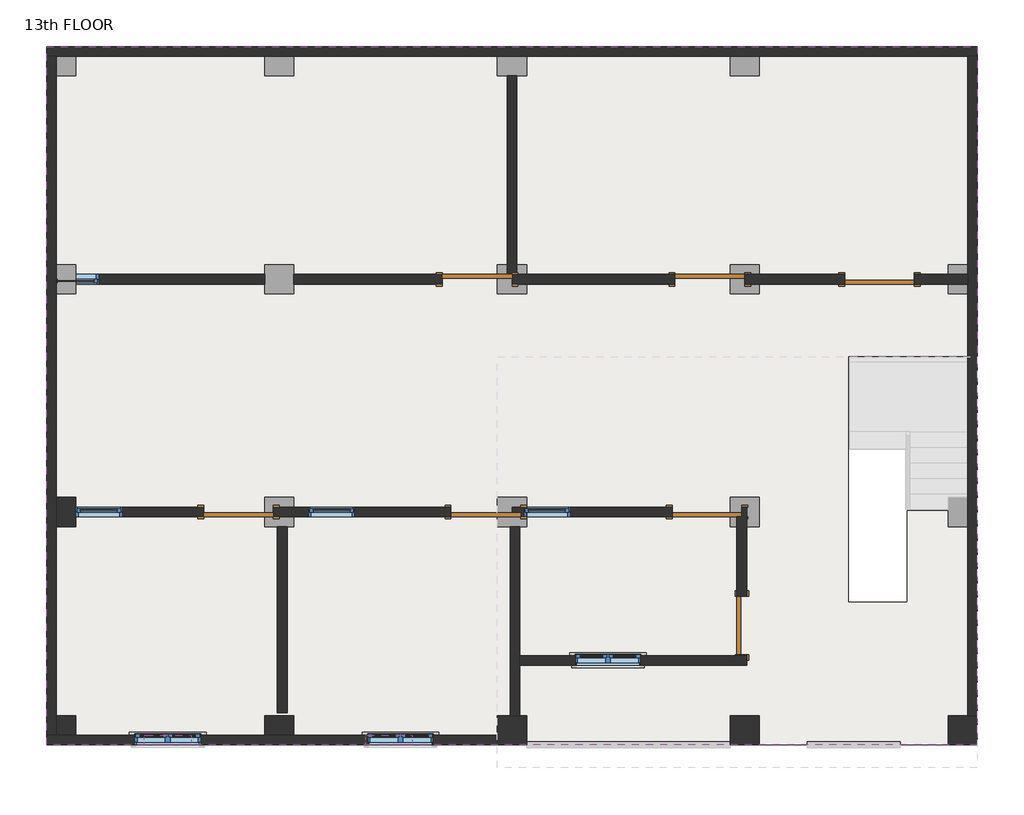
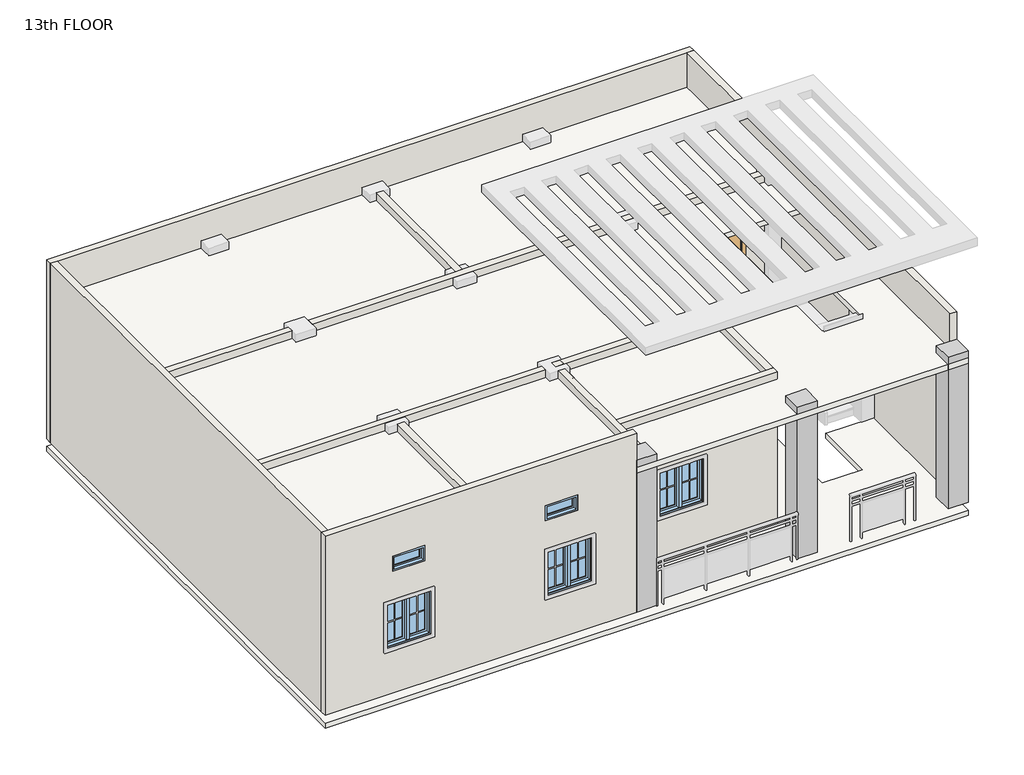
# One storey, part 1 of 2: 15 walls, 9 windows, 7 doors, 6 columns, 2 slabs.
"""IFC4 building model written with IfcOpenShell, lengths in millimetres."""

from ifc_helpers import new_model, si_unit, frame, origin, place, context, project, spatial, polyline, outline, extrude, faceted_brep, transform, mapped, element, save
from components import door_e00f436c, door_a1797ceb, window_4c2727af, window_0bf3737e, window_78893e6c, window_0d9958e7

model = new_model("IFC4")

# Units and contexts
model_context = context("Model", 3, world=origin())
ifc_project = project(units=[si_unit("LENGTHUNIT", "METRE", prefix="MILLI")], contexts=[model_context])

# Site, building, storey
site = spatial("IfcSite", under=ifc_project)
building = spatial("IfcBuilding", under=site)
storey = spatial("IfcBuildingStorey", under=building, Name="13th FLOOR", Elevation=39471.6)

# Columns
placement = place(None, origin())
element("IfcColumn", 1, ObjectType="column family : column family", at=placement, inside=storey, context=model_context, shape_type="SweptSolid", body=[
    extrude(outline(polyline([(-15433.597125, 2867.2065522), (-15433.597125, 2486.2065522), (-15687.597125, 2486.2065522), (-15687.597125, 2867.2065522), (-15433.597125, 2867.2065522)])), frame((0.0, 0.0, 39476.6), z_axis=(0.0, 0.0, 1.0), x_axis=(1.0, 0.0, 0.0)), (0.0, 0.0, 1.0), 3038.0),
])
element("IfcColumn", 2, ObjectType="column family : column family", at=placement, inside=storey, context=model_context, shape_type="SweptSolid", body=[
    extrude(outline(polyline([(-15433.597125, 9.7065522), (-15433.597125, -244.2934478), (-15687.597125, -244.2934478), (-15687.597125, 9.7065522), (-15433.597125, 9.7065522)])), frame((0.0, 0.0, 39476.6), z_axis=(0.0, 0.0, 1.0), x_axis=(1.0, 0.0, 0.0)), (0.0, 0.0, 1.0), 3038.0),
])
element("IfcColumn", 3, ObjectType="column family : column family", at=placement, inside=storey, context=model_context, shape_type="SweptSolid", body=[
    extrude(outline(polyline([(-3622.597125, 9.7065522), (-3622.597125, -371.2934478), (-4003.597125, -371.2934478), (-4003.597125, 9.7065522), (-3622.597125, 9.7065522)])), frame((0.0, 0.0, 39476.6), z_axis=(0.0, 0.0, 1.0), x_axis=(1.0, 0.0, 0.0)), (0.0, 0.0, 1.0), 3038.0),
])
element("IfcColumn", 4, ObjectType="column family : column family", at=placement, inside=storey, context=model_context, shape_type="SweptSolid", body=[
    extrude(outline(polyline([(-6480.097125, 9.7065522), (-6480.097125, -371.2934478), (-6861.097125, -371.2934478), (-6861.097125, 9.7065522), (-6480.097125, 9.7065522)])), frame((0.0, 0.0, 39476.6), z_axis=(0.0, 0.0, 1.0), x_axis=(1.0, 0.0, 0.0)), (0.0, 0.0, 1.0), 3038.0),
])
element("IfcColumn", 5, ObjectType="column family : column family", at=placement, inside=storey, context=model_context, shape_type="SweptSolid", body=[
    extrude(outline(polyline([(-9528.097125, 9.7065522), (-9528.097125, -371.2934478), (-9909.097125, -371.2934478), (-9909.097125, 9.7065522), (-9528.097125, 9.7065522)])), frame((0.0, 0.0, 39476.6), z_axis=(0.0, 0.0, 1.0), x_axis=(1.0, 0.0, 0.0)), (0.0, 0.0, 1.0), 3038.0),
])
element("IfcColumn", 6, ObjectType="column family : column family", at=placement, inside=storey, context=model_context, shape_type="SweptSolid", body=[
    extrude(outline(polyline([(-12957.097125, 9.7065522), (-12576.097125, 9.7065522), (-12576.097125, -244.2934478), (-12957.097125, -244.2934478), (-12957.097125, 9.7065522)])), frame((0.0, 0.0, 39476.6), z_axis=(0.0, 0.0, 1.0), x_axis=(1.0, 0.0, 0.0)), (0.0, 0.0, 1.0), 3038.0),
])

# Doors
door_shape = door_e00f436c(model_context)
element("IfcDoor", 7, ObjectType="Single-Flush : 30\" x 80\"", at=placement, inside=storey, context=model_context, shape_type="MappedRepresentation", body=[
    mapped(door_shape, transform((-6708.697125, 1190.8065522, 39471.6), x_axis=(0.0, -1.0, 0.0), y_axis=(1.0, 0.0, 0.0), z_axis=(0.0, 0.0, 1.0))),
])
door_2_shape = door_a1797ceb(model_context)
element("IfcDoor", 8, ObjectType="Single-Flush : 36\" x 84\"", at=placement, inside=storey, context=model_context, shape_type="MappedRepresentation", body=[
    mapped(door_2_shape, transform((-10175.797125, 5724.7065522, 39471.6), x_axis=(1.0, 0.0, 0.0), y_axis=(0.0, 1.0, 0.0), z_axis=(0.0, 0.0, 1.0))),
])
element("IfcDoor", 9, ObjectType="Single-Flush : 36\" x 84\"", at=placement, inside=storey, context=model_context, shape_type="MappedRepresentation", body=[
    mapped(door_2_shape, transform((-10061.497125, 2676.7065522, 39471.6), x_axis=(-1.0, 0.0, 0.0), y_axis=(0.0, -1.0, 0.0), z_axis=(0.0, 0.0, 1.0))),
])
element("IfcDoor", 10, ObjectType="Single-Flush : 36\" x 84\"", at=placement, inside=storey, context=model_context, shape_type="MappedRepresentation", body=[
    mapped(door_2_shape, transform((-13299.997125, 2676.7065522, 39471.6), x_axis=(-1.0, 0.0, 0.0), y_axis=(0.0, -1.0, 0.0), z_axis=(0.0, 0.0, 1.0))),
])
element("IfcDoor", 11, ObjectType="Single-Flush : 36\" x 84\"", at=placement, inside=storey, context=model_context, shape_type="MappedRepresentation", body=[
    mapped(door_2_shape, transform((-7127.797125, 5724.7065522, 39471.6), x_axis=(1.0, 0.0, 0.0), y_axis=(0.0, 1.0, 0.0), z_axis=(0.0, 0.0, 1.0))),
])
element("IfcDoor", 12, ObjectType="Single-Flush : 36\" x 84\"", at=placement, inside=storey, context=model_context, shape_type="MappedRepresentation", body=[
    mapped(door_2_shape, transform((-7165.897125, 2676.7065522, 39471.6), x_axis=(-1.0, 0.0, 0.0), y_axis=(0.0, -1.0, 0.0), z_axis=(0.0, 0.0, 1.0))),
])
element("IfcDoor", 13, ObjectType="Single-Flush : 36\" x 84\"", at=placement, inside=storey, context=model_context, shape_type="MappedRepresentation", body=[
    mapped(door_2_shape, transform((-4905.297125, 5724.7065522, 39471.6), x_axis=(-1.0, 0.0, 0.0), y_axis=(0.0, -1.0, 0.0), z_axis=(0.0, 0.0, 1.0))),
])

# Slabs
element("IfcSlab", 14, ObjectType="Generic - 4\"", at=placement, inside=storey, context=model_context, shape_type="SweptSolid", body=[
    extrude(outline(polyline([(-3622.597125, 8772.7065522), (-3622.597125, -371.2934478), (-15814.597125, -371.2934478), (-15814.597125, 8772.7065522), (-3622.597125, 8772.7065522)]), holes=[polyline([(-3734.357125, 4711.0719226), (-5310.2646464, 4711.0719226), (-5310.2646464, 1502.3126957), (-4547.7736682, 1502.3126957), (-4547.7736682, 2699.911213), (-3734.357125, 2699.911213), (-3734.357125, 4711.0719226)])]), frame((0.0, 0.0, 39217.6), z_axis=(0.0, 0.0, 1.0), x_axis=(1.0, 0.0, 0.0)), (0.0, 0.0, 1.0), 101.6),
])
element("IfcSlab", 15, ObjectType="Generic - 4\"", at=placement, inside=storey, context=model_context, shape_type="SweptSolid", body=[
    extrude(outline(polyline([(-3622.597125, 8772.7065522), (-3622.597125, -371.2934478), (-15814.597125, -371.2934478), (-15814.597125, 8772.7065522), (-3622.597125, 8772.7065522)]), holes=[polyline([(-3734.357125, 4711.0719226), (-5310.2646464, 4711.0719226), (-5310.2646464, 1502.3126957), (-4547.7736682, 1502.3126957), (-4547.7736682, 2699.911213), (-3734.357125, 2699.911213), (-3734.357125, 4711.0719226)])]), frame((0.0, 0.0, 42265.6), z_axis=(0.0, 0.0, 1.0), x_axis=(1.0, 0.0, 0.0)), (0.0, 0.0, 1.0), 101.6),
])

# Walls
element("IfcWall", 16, ObjectType="Generic - 5\"", at=placement, inside=storey, context=model_context, shape_type="Brep", body=[
    faceted_brep([(-15814.597125, 8645.7065522, 39471.6), (-15687.597125, 8645.7065522, 39471.6), (-3749.597125, 8645.7065522, 39471.6), (-3622.597125, 8645.7065522, 39471.6), (-3622.597125, 8645.7065522, 43063.6342883), (-3749.597125, 8645.7065522, 43063.6342883), (-15687.597125, 8645.7065522, 43063.6342883), (-15814.597125, 8645.7065522, 43063.6342883), (-15814.597125, 8772.7065522, 39471.6), (-15814.597125, 8772.7065522, 43063.6342883), (-3622.597125, 8772.7065522, 43063.6342883), (-3622.597125, 8772.7065522, 39471.6)], [[[0, 1, 2, 3, 4, 5, 6, 7]], [[8, 9, 10, 11]], [[3, 2, 1, 0, 8, 11]], [[7, 6, 5, 4, 10, 9]], [[4, 3, 11, 10]], [[0, 7, 9, 8]]]),
])
element("IfcWall", 17, ObjectType="Generic - 5\"", at=placement, inside=storey, context=model_context, shape_type="Brep", body=[
    faceted_brep([(-3749.597125, 8645.7065522, 39471.6), (-3749.597125, 5788.2065522, 39471.6), (-3749.597125, 5661.2065522, 39471.6), (-3749.597125, 9.7065522, 39471.6), (-3749.597125, 9.7065522, 43063.6342883), (-3749.597125, 8645.7065522, 43063.6342883), (-3622.597125, 8645.7065522, 39471.6), (-3622.597125, 8645.7065522, 43063.6342883), (-3622.597125, 9.7065522, 43063.6342883), (-3622.597125, 9.7065522, 42514.6), (-3622.597125, 9.7065522, 39476.6), (-3622.597125, 9.7065522, 39471.6)], [[[0, 1, 2, 3, 4, 5]], [[6, 7, 8, 9, 10, 11]], [[3, 2, 1, 0, 6, 11]], [[4, 3, 11, 10, 9, 8]], [[5, 4, 8, 7]], [[0, 5, 7, 6]]]),
])
element("IfcWall", 18, ObjectType="Generic - 5\"", at=placement, inside=storey, context=model_context, shape_type="Brep", body=[
    faceted_brep([(-9909.097125, -244.2934478, 39471.6), (-15687.597125, -244.2934478, 39471.6), (-15814.597125, -244.2934478, 39471.6), (-15814.597125, -244.2934478, 43063.6342883), (-15687.597125, -244.2934478, 43063.6342883), (-9909.097125, -244.2934478, 43063.6342883), (-13795.297125, -244.2934478, 41300.4), (-14658.897125, -244.2934478, 41300.4), (-14658.897125, -244.2934478, 40386.0), (-13795.297125, -244.2934478, 40386.0), (-10747.297125, -244.2934478, 41300.4), (-11610.897125, -244.2934478, 41300.4), (-11610.897125, -244.2934478, 40386.0), (-10747.297125, -244.2934478, 40386.0), (-13922.297125, -244.2934478, 42214.8), (-14531.897125, -244.2934478, 42214.8), (-14531.897125, -244.2934478, 41910.0), (-13922.297125, -244.2934478, 41910.0), (-11026.697125, -244.2934478, 42214.8), (-11636.297125, -244.2934478, 42214.8), (-11636.297125, -244.2934478, 41910.0), (-11026.697125, -244.2934478, 41910.0), (-9909.097125, -371.2934478, 39471.6), (-9909.097125, -371.2934478, 39476.6), (-9909.097125, -371.2934478, 42514.6), (-9909.097125, -371.2934478, 43063.6342883), (-15814.597125, -371.2934478, 43063.6342883), (-15814.597125, -371.2934478, 39471.6), (-13795.297125, -371.2934478, 41300.4), (-13795.297125, -371.2934478, 40386.0), (-14658.897125, -371.2934478, 40386.0), (-14658.897125, -371.2934478, 41300.4), (-10747.297125, -371.2934478, 41300.4), (-10747.297125, -371.2934478, 40386.0), (-11610.897125, -371.2934478, 40386.0), (-11610.897125, -371.2934478, 41300.4), (-13922.297125, -371.2934478, 42214.8), (-13922.297125, -371.2934478, 41910.0), (-14531.897125, -371.2934478, 41910.0), (-14531.897125, -371.2934478, 42214.8), (-11026.697125, -371.2934478, 42214.8), (-11026.697125, -371.2934478, 41910.0), (-11636.297125, -371.2934478, 41910.0), (-11636.297125, -371.2934478, 42214.8)], [[[0, 1, 2, 3, 4, 5], [6, 7, 8, 9], [10, 11, 12, 13], [14, 15, 16, 17], [18, 19, 20, 21]], [[22, 23, 24, 25, 26, 27], [28, 29, 30, 31], [32, 33, 34, 35], [36, 37, 38, 39], [40, 41, 42, 43]], [[2, 1, 0, 22, 27]], [[5, 4, 3, 26, 25]], [[0, 5, 25, 24, 23, 22]], [[3, 2, 27, 26]], [[29, 28, 6, 9]], [[30, 29, 9, 8]], [[31, 30, 8, 7]], [[28, 31, 7, 6]], [[33, 32, 10, 13]], [[34, 33, 13, 12]], [[35, 34, 12, 11]], [[32, 35, 11, 10]], [[37, 36, 14, 17]], [[38, 37, 17, 16]], [[39, 38, 16, 15]], [[36, 39, 15, 14]], [[41, 40, 18, 21]], [[42, 41, 21, 20]], [[43, 42, 20, 19]], [[40, 43, 19, 18]]]),
])
element("IfcWall", 19, ObjectType="Generic - 5\"", at=placement, inside=storey, context=model_context, shape_type="Brep", body=[
    faceted_brep([(-15687.597125, -244.2934478, 39471.6), (-15687.597125, 8645.7065522, 39471.6), (-15687.597125, 8645.7065522, 39476.6), (-15687.597125, 8645.7065522, 42514.6), (-15687.597125, 8645.7065522, 43063.6342883), (-15687.597125, -244.2934478, 43063.6342883), (-15687.597125, -244.2934478, 42514.6), (-15687.597125, -244.2934478, 39476.6), (-15814.597125, -244.2934478, 39471.6), (-15814.597125, -244.2934478, 43063.6342883), (-15814.597125, 8645.7065522, 43063.6342883), (-15814.597125, 8645.7065522, 39471.6)], [[[0, 1, 2, 3, 4, 5, 6, 7]], [[8, 9, 10, 11]], [[1, 0, 8, 11]], [[5, 4, 10, 9]], [[4, 3, 2, 1, 11, 10]], [[0, 7, 6, 5, 9, 8]]]),
])
element("IfcWall", 20, ObjectType="Generic - 5\"", at=placement, inside=storey, context=model_context, shape_type="SweptSolid", body=[
    extrude(outline(polyline([(39471.6, -15433.597125), (39471.6, -12957.097125), (42519.6, -12957.097125), (42519.6, -15433.597125), (41605.2, -15433.597125), (41605.2, -15128.797125), (39776.4, -15128.797125), (39776.4, -15433.597125), (39471.6, -15433.597125)])), frame((0.0, 5661.2065522, 0.0), z_axis=(0.0, 1.0, 0.0), x_axis=(0.0, 0.0, 1.0)), (0.0, 0.0, 1.0), 127.0),
])
element("IfcWall", 21, ObjectType="Generic - 5\"", at=placement, inside=storey, context=model_context, shape_type="Brep", body=[
    faceted_brep([(-9782.097125, 8391.7065522, 39471.6), (-9782.097125, 5788.2065522, 39471.6), (-9782.097125, 5788.2065522, 39476.6), (-9782.097125, 5788.2065522, 41605.2), (-9782.097125, 5788.2065522, 42514.6), (-9782.097125, 5788.2065522, 42519.6), (-9782.097125, 8391.7065522, 42519.6), (-9655.097125, 8391.7065522, 39471.6), (-9655.097125, 8391.7065522, 42519.6), (-9655.097125, 5788.2065522, 42519.6), (-9655.097125, 5788.2065522, 42514.6), (-9655.097125, 5788.2065522, 39476.6), (-9655.097125, 5788.2065522, 39471.6), (-9718.597125, 5788.2065522, 39471.6)], [[[0, 1, 2, 3, 4, 5, 6]], [[7, 8, 9, 10, 11, 12]], [[1, 0, 7, 12, 13]], [[6, 5, 9, 8]], [[0, 6, 8, 7]], [[5, 4, 3, 2, 1, 13, 12, 11, 10, 9]]]),
])
element("IfcWall", 22, ObjectType="Generic - 5\"", at=placement, inside=storey, context=model_context, shape_type="Brep", body=[
    faceted_brep([(-6670.597125, 5661.2065522, 39471.6), (-5362.497125, 5661.2065522, 39471.6), (-5362.497125, 5661.2065522, 41605.2), (-4448.097125, 5661.2065522, 41605.2), (-4448.097125, 5661.2065522, 39471.6), (-3749.597125, 5661.2065522, 39471.6), (-3749.597125, 5661.2065522, 39476.6), (-3749.597125, 5661.2065522, 42514.6), (-3749.597125, 5661.2065522, 42519.6), (-12576.097125, 5661.2065522, 42519.6), (-12576.097125, 5661.2065522, 39471.6), (-10632.997125, 5661.2065522, 39471.6), (-10632.997125, 5661.2065522, 41605.2), (-9909.097125, 5661.2065522, 41605.2), (-9718.597125, 5661.2065522, 41605.2), (-9718.597125, 5661.2065522, 39476.6), (-9718.597125, 5661.2065522, 39471.6), (-7584.997125, 5661.2065522, 39471.6), (-7584.997125, 5661.2065522, 41605.2), (-6861.097125, 5661.2065522, 41605.2), (-6670.597125, 5661.2065522, 41605.2), (-6670.597125, 5661.2065522, 39476.6), (-5362.497125, 5788.2065522, 41605.2), (-5362.497125, 5788.2065522, 39471.6), (-6670.597125, 5788.2065522, 39471.6), (-6670.597125, 5788.2065522, 39476.6), (-6670.597125, 5788.2065522, 41605.2), (-6861.097125, 5788.2065522, 41605.2), (-7584.997125, 5788.2065522, 41605.2), (-7584.997125, 5788.2065522, 39471.6), (-9655.097125, 5788.2065522, 39471.6), (-9718.597125, 5788.2065522, 39471.6), (-9718.597125, 5788.2065522, 39476.6), (-9718.597125, 5788.2065522, 41605.2), (-9782.097125, 5788.2065522, 41605.2), (-9909.097125, 5788.2065522, 41605.2), (-10632.997125, 5788.2065522, 41605.2), (-10632.997125, 5788.2065522, 39471.6), (-12576.097125, 5788.2065522, 39471.6), (-12576.097125, 5788.2065522, 42519.6), (-9782.097125, 5788.2065522, 42519.6), (-9655.097125, 5788.2065522, 42519.6), (-3749.597125, 5788.2065522, 42519.6), (-3749.597125, 5788.2065522, 42514.6), (-3749.597125, 5788.2065522, 39476.6), (-3749.597125, 5788.2065522, 39471.6), (-4448.097125, 5788.2065522, 39471.6), (-4448.097125, 5788.2065522, 41605.2)], [[[0, 1, 2, 3, 4, 5, 6, 7, 8, 9, 10, 11, 12, 13, 14, 15, 16, 17, 18, 19, 20, 21]], [[22, 23, 24, 25, 26, 27, 28, 29, 30, 31, 32, 33, 34, 35, 36, 37, 38, 39, 40, 41, 42, 43, 44, 45, 46, 47]], [[11, 10, 38, 37]], [[17, 16, 31, 30, 29]], [[46, 45, 5, 4]], [[24, 23, 1, 0]], [[9, 8, 42, 41, 40, 39]], [[10, 9, 39, 38]], [[8, 7, 6, 5, 45, 44, 43, 42]], [[33, 32, 31, 16, 15, 14]], [[36, 35, 34, 33, 14, 13, 12]], [[37, 36, 12, 11]], [[26, 25, 24, 0, 21, 20]], [[28, 27, 26, 20, 19, 18]], [[29, 28, 18, 17]], [[2, 1, 23, 22]], [[3, 2, 22, 47]], [[4, 3, 47, 46]]]),
])
element("IfcWall", 23, ObjectType="Generic - 5\"", at=placement, inside=storey, context=model_context, shape_type="Brep", body=[
    faceted_brep([(-14823.997125, 2613.2065522, 39776.4), (-15433.597125, 2613.2065522, 39776.4), (-15433.597125, 2613.2065522, 39471.6), (-13757.197125, 2613.2065522, 39471.6), (-13757.197125, 2613.2065522, 41605.2), (-12957.097125, 2613.2065522, 41605.2), (-12842.797125, 2613.2065522, 41605.2), (-12842.797125, 2613.2065522, 39476.6), (-12842.797125, 2613.2065522, 39471.6), (-10518.697125, 2613.2065522, 39471.6), (-10518.697125, 2613.2065522, 41605.2), (-9909.097125, 2613.2065522, 41605.2), (-9909.097125, 2613.2065522, 42519.6), (-15433.597125, 2613.2065522, 42519.6), (-15433.597125, 2613.2065522, 41605.2), (-14823.997125, 2613.2065522, 41605.2), (-12385.597125, 2613.2065522, 41605.2), (-11775.997125, 2613.2065522, 41605.2), (-11775.997125, 2613.2065522, 39776.4), (-12385.597125, 2613.2065522, 39776.4), (-15433.597125, 2740.2065522, 39471.6), (-15433.597125, 2740.2065522, 39776.4), (-14823.997125, 2740.2065522, 39776.4), (-14823.997125, 2740.2065522, 41605.2), (-15433.597125, 2740.2065522, 41605.2), (-15433.597125, 2740.2065522, 42519.6), (-9909.097125, 2740.2065522, 42519.6), (-9909.097125, 2740.2065522, 41605.2), (-10518.697125, 2740.2065522, 41605.2), (-10518.697125, 2740.2065522, 39471.6), (-12842.797125, 2740.2065522, 39471.6), (-12842.797125, 2740.2065522, 39476.6), (-12842.797125, 2740.2065522, 41605.2), (-12957.097125, 2740.2065522, 41605.2), (-13757.197125, 2740.2065522, 41605.2), (-13757.197125, 2740.2065522, 39471.6), (-12385.597125, 2740.2065522, 41605.2), (-12385.597125, 2740.2065522, 39776.4), (-11775.997125, 2740.2065522, 39776.4), (-11775.997125, 2740.2065522, 41605.2)], [[[0, 1, 2, 3, 4, 5, 6, 7, 8, 9, 10, 11, 12, 13, 14, 15], [16, 17, 18, 19]], [[20, 21, 22, 23, 24, 25, 26, 27, 28, 29, 30, 31, 32, 33, 34, 35], [36, 37, 38, 39]], [[30, 29, 9, 8]], [[20, 35, 3, 2]], [[26, 12, 11, 27]], [[13, 12, 26, 25]], [[14, 13, 25, 24]], [[2, 1, 21, 20]], [[28, 10, 9, 29]], [[10, 28, 27, 11]], [[4, 3, 35, 34]], [[6, 5, 4, 34, 33, 32]], [[8, 7, 6, 32, 31, 30]], [[22, 21, 1, 0]], [[23, 22, 0, 15]], [[24, 23, 15, 14]], [[37, 36, 16, 19]], [[38, 37, 19, 18]], [[39, 38, 18, 17]], [[36, 39, 17, 16]]]),
])
element("IfcWall", 24, ObjectType="Generic - 5\"", at=placement, inside=storey, context=model_context, shape_type="Brep", body=[
    faceted_brep([(-9616.997125, 9.7065522, 39471.6), (-9616.997125, 670.1065522, 39471.6), (-9616.997125, 797.1065522, 39471.6), (-9616.997125, 2486.2065522, 39471.6), (-9616.997125, 2486.2065522, 42519.6), (-9616.997125, 797.1065522, 42519.6), (-9616.997125, 670.1065522, 42519.6), (-9616.997125, 9.7065522, 42519.6), (-9743.997125, 9.7065522, 39471.6), (-9743.997125, 9.7065522, 42519.6), (-9743.997125, 2486.2065522, 42519.6), (-9743.997125, 2486.2065522, 39471.6)], [[[0, 1, 2, 3, 4, 5, 6, 7]], [[8, 9, 10, 11]], [[3, 2, 1, 0, 8, 11]], [[4, 3, 11, 10]], [[7, 6, 5, 4, 10, 9]], [[0, 7, 9, 8]]]),
])
element("IfcWall", 25, ObjectType="Generic - 5\"", at=placement, inside=storey, context=model_context, shape_type="SweptSolid", body=[
    extrude(outline(polyline([(-9743.997125, 2181.4065522), (-9743.997125, 2486.2065522), (-9616.997125, 2486.2065522), (-9616.997125, 2181.4065522), (-9743.997125, 2181.4065522)])), frame((0.0, 0.0, 39471.6), z_axis=(0.0, 0.0, 1.0), x_axis=(1.0, 0.0, 0.0)), (0.0, 0.0, 1.0), 3048.0),
])
element("IfcWall", 26, ObjectType="Generic - 5\"", at=placement, inside=storey, context=model_context, shape_type="Brep", body=[
    faceted_brep([(-6772.197125, 2613.2065522, 42519.6), (-9718.597125, 2613.2065522, 42519.6), (-9718.597125, 2613.2065522, 42514.6), (-9718.597125, 2613.2065522, 39476.6), (-9718.597125, 2613.2065522, 39471.6), (-7623.097125, 2613.2065522, 39471.6), (-7623.097125, 2613.2065522, 41605.2), (-6861.097125, 2613.2065522, 41605.2), (-6772.197125, 2613.2065522, 41605.2), (-6772.197125, 2613.2065522, 42514.6), (-9566.197125, 2613.2065522, 41605.2), (-9528.097125, 2613.2065522, 41605.2), (-8956.597125, 2613.2065522, 41605.2), (-8956.597125, 2613.2065522, 39776.4), (-9528.097125, 2613.2065522, 39776.4), (-9566.197125, 2613.2065522, 39776.4), (-9718.597125, 2740.2065522, 42519.6), (-6772.197125, 2740.2065522, 42519.6), (-6772.197125, 2740.2065522, 41605.2), (-6861.097125, 2740.2065522, 41605.2), (-7623.097125, 2740.2065522, 41605.2), (-7623.097125, 2740.2065522, 39471.6), (-9718.597125, 2740.2065522, 39471.6), (-9718.597125, 2740.2065522, 39476.6), (-9718.597125, 2740.2065522, 42514.6), (-9566.197125, 2740.2065522, 41605.2), (-9566.197125, 2740.2065522, 39776.4), (-9528.097125, 2740.2065522, 39776.4), (-8956.597125, 2740.2065522, 39776.4), (-8956.597125, 2740.2065522, 41605.2), (-9528.097125, 2740.2065522, 41605.2)], [[[0, 1, 2, 3, 4, 5, 6, 7, 8, 9], [10, 11, 12, 13, 14, 15]], [[16, 17, 18, 19, 20, 21, 22, 23, 24], [25, 26, 27, 28, 29, 30]], [[4, 22, 21, 5]], [[1, 0, 17, 16]], [[4, 3, 2, 1, 16, 24, 23, 22]], [[26, 25, 10, 15]], [[28, 27, 26, 15, 14, 13]], [[29, 28, 13, 12]], [[25, 30, 29, 12, 11, 10]], [[20, 6, 5, 21]], [[6, 20, 19, 18, 8, 7]], [[17, 0, 9, 8, 18]]]),
])
element("IfcWall", 27, ObjectType="Generic - 5\"", at=placement, inside=storey, context=model_context, shape_type="Brep", body=[
    faceted_brep([(-6645.197125, 797.1065522, 39471.6), (-6645.197125, 809.8065522, 39471.6), (-6645.197125, 809.8065522, 41503.6), (-6645.197125, 1571.8065522, 41503.6), (-6645.197125, 1571.8065522, 39471.6), (-6645.197125, 2740.2065522, 39471.6), (-6645.197125, 2740.2065522, 39476.6), (-6645.197125, 2740.2065522, 42514.6), (-6645.197125, 2740.2065522, 42519.6), (-6645.197125, 797.1065522, 42519.6), (-6772.197125, 809.8065522, 41503.6), (-6772.197125, 809.8065522, 39471.6), (-6772.197125, 797.1065522, 39471.6), (-6772.197125, 797.1065522, 42519.6), (-6772.197125, 2613.2065522, 42519.6), (-6772.197125, 2740.2065522, 42519.6), (-6772.197125, 2740.2065522, 41605.2), (-6772.197125, 2613.2065522, 41605.2), (-6772.197125, 2613.2065522, 39476.6), (-6772.197125, 2613.2065522, 39471.6), (-6772.197125, 1571.8065522, 39471.6), (-6772.197125, 1571.8065522, 41503.6), (-6708.697125, 2613.2065522, 39471.6), (-6708.697125, 2740.2065522, 39471.6), (-6708.697125, 2613.2065522, 41605.2), (-6708.697125, 2613.2065522, 39476.6), (-6708.697125, 2740.2065522, 41605.2), (-6708.697125, 2740.2065522, 39476.6)], [[[0, 1, 2, 3, 4, 5, 6, 7, 8, 9]], [[10, 11, 12, 13, 14, 15, 16, 17, 18, 19, 20, 21]], [[20, 19, 22, 23, 5, 4]], [[12, 11, 1, 0]], [[9, 8, 15, 14, 13]], [[24, 25, 22, 19, 18, 17]], [[26, 24, 17, 16]], [[22, 25, 24, 26, 27, 23]], [[8, 7, 6, 5, 23, 27, 26, 16, 15]], [[0, 9, 13, 12]], [[2, 1, 11, 10]], [[3, 2, 10, 21]], [[4, 3, 21, 20]]]),
])
element("IfcWall", 28, ObjectType="Generic - 5\"", at=placement, inside=storey, context=model_context, shape_type="Brep", body=[
    faceted_brep([(-9718.597125, 2613.2065522, 39471.6), (-9566.197125, 2613.2065522, 39471.6), (-9566.197125, 2613.2065522, 39776.4), (-9566.197125, 2613.2065522, 41605.2), (-9566.197125, 2613.2065522, 42519.6), (-9718.597125, 2613.2065522, 42519.6), (-9718.597125, 2613.2065522, 42514.6), (-9718.597125, 2613.2065522, 39476.6), (-9718.597125, 2740.2065522, 39471.6), (-9718.597125, 2740.2065522, 39476.6), (-9718.597125, 2740.2065522, 42514.6), (-9718.597125, 2740.2065522, 42519.6), (-9566.197125, 2740.2065522, 42519.6), (-9566.197125, 2740.2065522, 41605.2), (-9566.197125, 2740.2065522, 39776.4), (-9566.197125, 2740.2065522, 39471.6)], [[[0, 1, 2, 3, 4, 5, 6, 7]], [[8, 9, 10, 11, 12, 13, 14, 15]], [[1, 0, 8, 15]], [[4, 3, 2, 1, 15, 14, 13, 12]], [[5, 4, 12, 11]], [[0, 7, 6, 5, 11, 10, 9, 8]]]),
])
element("IfcWall", 29, ObjectType="Generic - 5\"", at=placement, inside=storey, context=model_context, shape_type="SweptSolid", body=[
    extrude(outline(polyline([(-12791.997125, 47.8065522), (-12791.997125, 2486.2065522), (-12664.997125, 2486.2065522), (-12664.997125, 47.8065522), (-12791.997125, 47.8065522)])), frame((0.0, 0.0, 39471.6), z_axis=(0.0, 0.0, 1.0), x_axis=(1.0, 0.0, 0.0)), (0.0, 0.0, 1.0), 3048.0),
])
element("IfcWall", 30, ObjectType="Generic - 5\"", at=placement, inside=storey, context=model_context, shape_type="Brep", body=[
    faceted_brep([(-9616.997125, 670.1065522, 39471.6), (-6645.197125, 670.1065522, 39471.6), (-6645.197125, 670.1065522, 42519.6), (-9616.997125, 670.1065522, 42519.6), (-8029.497125, 670.1065522, 41300.4), (-8029.497125, 670.1065522, 40386.0), (-8893.097125, 670.1065522, 40386.0), (-8893.097125, 670.1065522, 41300.4), (-9616.997125, 797.1065522, 39471.6), (-9616.997125, 797.1065522, 42519.6), (-6772.197125, 797.1065522, 42519.6), (-6645.197125, 797.1065522, 42519.6), (-6645.197125, 797.1065522, 39471.6), (-6772.197125, 797.1065522, 39471.6), (-8029.497125, 797.1065522, 41300.4), (-8893.097125, 797.1065522, 41300.4), (-8893.097125, 797.1065522, 40386.0), (-8029.497125, 797.1065522, 40386.0)], [[[0, 1, 2, 3], [4, 5, 6, 7]], [[8, 9, 10, 11, 12, 13], [14, 15, 16, 17]], [[1, 0, 8, 13, 12]], [[3, 2, 11, 10, 9]], [[0, 3, 9, 8]], [[2, 1, 12, 11]], [[5, 4, 14, 17]], [[6, 5, 17, 16]], [[7, 6, 16, 15]], [[4, 7, 15, 14]]]),
])

# Windows
window_shape = window_4c2727af(model_context)
element("IfcWindow", 31, ObjectType="Fixed : 24\" x 12\"", at=placement, inside=storey, context=model_context, shape_type="MappedRepresentation", body=[
    mapped(window_shape, transform((-14188.997125, -307.7934478, 40995.6), x_axis=(1.0, 0.0, 0.0), y_axis=(0.0, 1.0, 0.0), z_axis=(0.0, 0.0, 1.0))),
])
element("IfcWindow", 32, ObjectType="Fixed : 24\" x 12\"", at=placement, inside=storey, context=model_context, shape_type="MappedRepresentation", body=[
    mapped(window_shape, transform((-11293.397125, -307.7934478, 40995.6), x_axis=(1.0, 0.0, 0.0), y_axis=(0.0, 1.0, 0.0), z_axis=(0.0, 0.0, 1.0))),
])
window_2_shape = window_0bf3737e(model_context)
element("IfcWindow", 33, ObjectType="Fixed : 24\" x 72\"", at=placement, inside=storey, context=model_context, shape_type="MappedRepresentation", body=[
    mapped(window_2_shape, transform((-15471.697125, 5724.7065522, 39471.6), x_axis=(-1.0, 0.0, 0.0), y_axis=(0.0, -1.0, 0.0), z_axis=(0.0, 0.0, 1.0))),
])
window_3_shape = window_78893e6c(model_context)
element("IfcWindow", 34, ObjectType="Fixed : 24\" x 72\"", at=placement, inside=storey, context=model_context, shape_type="MappedRepresentation", body=[
    mapped(window_3_shape, transform((-15166.897125, 2676.7065522, 39471.6), x_axis=(-1.0, 0.0, 0.0), y_axis=(0.0, -1.0, 0.0), z_axis=(0.0, 0.0, 1.0))),
])
element("IfcWindow", 35, ObjectType="Fixed : 24\" x 72\"", at=placement, inside=storey, context=model_context, shape_type="MappedRepresentation", body=[
    mapped(window_3_shape, transform((-12118.897125, 2676.7065522, 39471.6), x_axis=(-1.0, 0.0, 0.0), y_axis=(0.0, -1.0, 0.0), z_axis=(0.0, 0.0, 1.0))),
])
element("IfcWindow", 36, ObjectType="Fixed : 24\" x 72\"", at=placement, inside=storey, context=model_context, shape_type="MappedRepresentation", body=[
    mapped(window_3_shape, transform((-9299.497125, 2676.7065522, 39471.6), x_axis=(-1.0, 0.0, 0.0), y_axis=(0.0, -1.0, 0.0), z_axis=(0.0, 0.0, 1.0))),
])
window_4_shape = window_0d9958e7(model_context)
element("IfcWindow", 37, ObjectType="Window-Casement-Double : 34\" x 36\"", at=placement, inside=storey, context=model_context, shape_type="MappedRepresentation", body=[
    mapped(window_4_shape, transform((-14227.097125, -307.7934478, 39471.6), x_axis=(1.0, 0.0, 0.0), y_axis=(0.0, 1.0, 0.0), z_axis=(0.0, 0.0, 1.0))),
])
element("IfcWindow", 38, ObjectType="Window-Casement-Double : 34\" x 36\"", at=placement, inside=storey, context=model_context, shape_type="MappedRepresentation", body=[
    mapped(window_4_shape, transform((-11179.097125, -307.7934478, 39471.6), x_axis=(1.0, 0.0, 0.0), y_axis=(0.0, 1.0, 0.0), z_axis=(0.0, 0.0, 1.0))),
])
element("IfcWindow", 39, ObjectType="Window-Casement-Double : 34\" x 36\"", at=placement, inside=storey, context=model_context, shape_type="MappedRepresentation", body=[
    mapped(window_4_shape, transform((-8461.297125, 733.6065522, 39471.6), x_axis=(1.0, 0.0, 0.0), y_axis=(0.0, 1.0, 0.0), z_axis=(0.0, 0.0, 1.0))),
])

save(model, "model.ifc")

# Revit data of these elements
# Type "column family : column family"
#   w2 [instance default] = 0' - 9.88189"
#   w1 [instance default] = 0' - 9.01575"
#   Depth = 1' - 11.62205"
#   Width = 1' - 11.62205"
# Type "Single-Flush : 30\" x 80\""
#   Type Mark = "5"
#   Construction Type Id = "MDOOR"
#   Assembly Code = "C1020"
#   Analytic Construction = "Metal"
#   Thickness = 0' - 2"
#   Heat Transfer Coefficient (U) = 0.651978 BTU/(h·ft²·°F)
#   Height = 6' - 8"
#   Trim Projection Ext = 0' - 1"
#   Trim Projection Int = 0' - 1"
#   Trim Width = 0' - 3"
#   Width = 2' - 6"
#   Define Thermal Properties by = 1
#   Define Thermal Properties by = 1
#   Door Material = Door - Panel
#   Frame Material = Door - Frame
#   Visual Light Transmittance = 0
#   Solar Heat Gain Coefficient = 0
#   Function = (empty or 0)
#   Wall Closure = (empty or 0)
# Type "Single-Flush : 36\" x 84\""
#   Type Mark = "1"
#   Construction Type Id = "MDOOR"
#   Assembly Code = "C1020"
#   Analytic Construction = "Metal"
#   Thickness = 0' - 2"
#   Heat Transfer Coefficient (U) = 0.651978 BTU/(h·ft²·°F)
#   Height = 7' - 0"
#   Trim Projection Ext = 0' - 1"
#   Trim Projection Int = 0' - 1"
#   Trim Width = 0' - 3"
#   Width = 3' - 0"
#   Define Thermal Properties by = 1
#   Define Thermal Properties by = 1
#   Door Material = Door - Panel
#   Frame Material = Door - Frame
#   Visual Light Transmittance = 0
#   Solar Heat Gain Coefficient = 0
#   Function = (empty or 0)
#   Wall Closure = (empty or 0)
# Type "Generic - 4\""
#   Assembly Code = "B1010"
#   Function = 0
#   Layers, outside or top first: 0' - 4" no material (function 1)
# Type "Generic - 5\""
#   Assembly Code = "B2010"
#   Layers, outside or top first: 0' - 5" no material (function 1)
# Type "Fixed : 24\" x 12\""
#   Type Mark = "4"
#   Construction Type Id = "GSP4R"
#   Assembly Code = "B2020100"
#   Analytic Construction = "1/8 in Pilkington single glazing"
#   Visual Light Transmittance = 0.9
#   Solar Heat Gain Coefficient = 0.78
#   Heat Transfer Coefficient (U) = 0.6496 BTU/(h·ft²·°F)
#   Height = 1' - 0"
#   Default Sill Height = 3' - 0"
#   Width = 2' - 0"
#   Window Inset = 0' - 0 3/4"
#   Define Thermal Properties by = 1
#   Define Thermal Properties by = 1
#   Glass Pane Material = Glass
#   Sash Material = Sash
#   Wall Closure = (empty or 0)
# Type "Fixed : 24\" x 72\""
#   Type Mark = "7"
#   Construction Type Id = "GSP4R"
#   Assembly Code = "B2020100"
#   Analytic Construction = "1/8 in Pilkington single glazing"
#   Visual Light Transmittance = 0.9
#   Solar Heat Gain Coefficient = 0.78
#   Heat Transfer Coefficient (U) = 0.6496 BTU/(h·ft²·°F)
#   Height = 6' - 0"
#   Default Sill Height = 1' - 0"
#   Width = 2' - 0"
#   Window Inset = 0' - 0 3/4"
#   Define Thermal Properties by = 1
#   Define Thermal Properties by = 1
#   Glass Pane Material = Glass
#   Sash Material = Sash
#   Wall Closure = (empty or 0)
# Type "Window-Casement-Double : 34\" x 36\""
#   Type Mark = "14"
#   Fire Rating = "0.5h"
#   Assembly Code = "B2020100"
#   Analytic Construction = "Double glazing - domestic"
#   Frame Extension [instance default] = 0' - 0 1/4"
#   Window Inset [instance default] = 0' - 0"
#   Wall Thickness [instance default] = 0' - 6"
#   Interior Wall Closure [instance default] = 0' - 2 1/4"
#   Half Width = 1' - 5"
#   Visual Light Transmittance = 0.81
#   Thermal Resistance (R) = 1.8146 (h·ft²·°F)/BTU
#   Solar Heat Gain Coefficient = 0.76
#   Rough Width = 2' - 10 1/2"
#   Rough Height = 3' - 0 1/2"
#   Height = 3' - 0"
#   Heat Transfer Coefficient (U) = 0.5511 BTU/(h·ft²·°F)
#   Exterior Wall Closure [instance default] = 0' - 1 1/4"
#   Extension Jamb [instance default] = 0' - 2 1/4"
#   Default Sill Height = 3' - 0"
#   Width = 2' - 10"
#   Define Thermal Properties by = 0
#   Muntin Visibility = yes
#   Interior Trim Visibility [instance default] = yes
#   Exterior Trim Visibility [instance default] = yes
#   Extension Jamb Visibility [instance default] = yes
#   Interior Trim Material = Wood - Stained
#   Muntin Pattern = Muntin Pattern_2x2 : Muntin Pattern_2x2
#   Interior Trim = Trim-Window-Interior-Flat : Picture Frame
#   Interior Frame Material = Wood - Stained
#   Glass Panel Material = Glass
#   Exterior Trim Material = Clad - White
#   Exterior Trim = Trim-Window-Exterior-Flat : with Sill
#   Exterior Frame Material = Clad - White
#   Wall Closure = (empty or 0)
# Element 1 (IfcColumn, "column family : column family")
#   w2 = 1' - 3"
#   w1 = 0' - 10"
#   Phase Created = New Construction
#   Materials on its faces: "inside wall", "Default Wall"
# Elements 2, 6 (IfcColumn, "column family : column family")
#   w2 = 1' - 3"
#   w1 = 1' - 3"
#   Phase Created = New Construction
#   Materials on its faces: "Default Wall"
# Element 3 (IfcColumn, "column family : column family")
#   w2 = 1' - 3"
#   w1 = 1' - 3"
#   Phase Created = New Construction
#   Materials on its faces: "Clad - White", "Default Wall"
# Element 4 (IfcColumn, "column family : column family")
#   w2 = 1' - 3"
#   w1 = 1' - 3"
#   Phase Created = New Construction
#   Materials on its faces: "out side wall"
# Element 5 (IfcColumn, "column family : column family")
#   w2 = 1' - 3"
#   w1 = 1' - 3"
#   Phase Created = New Construction
#   Materials on its faces: "out side wall", "Default Wall"
# Element 7 (IfcDoor, "Single-Flush : 30\" x 80\"")
#   Phase Created = New Construction
#   Materials on its faces: "Door - Frame", "Door - Panel"
# Elements 8, 9, 10, 11, 12, 13 (IfcDoor, "Single-Flush : 36\" x 84\"")
#   Phase Created = New Construction
#   Materials on its faces: "Door - Frame", "Door - Panel"
# Element 14 (IfcSlab, "Generic - 4\"")
#   Height Offset From Level = -0' - 6"
#   Phase Created = New Construction
#   Materials on its faces: "Default Floor", "Clad - White", "floor"
# Element 15 (IfcSlab, "Generic - 4\"")
#   Height Offset From Level = 9' - 6"
#   Phase Created = New Construction
#   Materials on its faces: "Default Floor", "Clad - White"
# Element 16 (IfcWall, "Generic - 5\"")
#   Top Offset = 11' - 9.41867"
#   Base Offset = 0' - 0"
#   wall height = 11' - 9.41867"
#   Phase Created = New Construction
#   Base Constraint = 13th FLOOR
#   Top Constraint = 13th FLOOR
#   Materials on its faces: "Default Wall", "Clad - White"
# Element 17 (IfcWall, "Generic - 5\"")
#   Top Offset = 11' - 9.41867"
#   Base Offset = 0' - 0"
#   wall height = 11' - 9.41867"
#   Phase Created = New Construction
#   Base Constraint = 13th FLOOR
#   Top Constraint = 13th FLOOR
#   Materials on its faces: "Default Wall", "grey", "Clad - White"
# Element 18 (IfcWall, "Generic - 5\"")
#   Top Offset = 11' - 9.41867"
#   Base Offset = 0' - 0"
#   wall height = 11' - 9.41867"
#   Phase Created = New Construction
#   Base Constraint = 13th FLOOR
#   Top Constraint = 13th FLOOR
#   Materials on its faces: "Default Wall", "out side wall", "Clad - White"
# Element 19 (IfcWall, "Generic - 5\"")
#   Top Offset = 11' - 9.41867"
#   Base Offset = 0' - 0"
#   wall height = 11' - 9.41867"
#   Phase Created = New Construction
#   Base Constraint = 13th FLOOR
#   Top Constraint = 13th FLOOR
#   Materials on its faces: "Default Wall", "inside wall", "Clad - White"
# Elements 20, 23, 26 (IfcWall, "Generic - 5\"")
#   Top Offset = 10' - 0"
#   Base Offset = 0' - 0"
#   wall height = 10' - 0"
#   Phase Created = New Construction
#   Base Constraint = 13th FLOOR
#   Top Constraint = 13th FLOOR
#   Materials on its faces: "Default Wall", "inside wall"
# Elements 21, 25, 28, 29 (IfcWall, "Generic - 5\"")
#   Top Offset = 10' - 0"
#   Base Offset = 0' - 0"
#   wall height = 10' - 0"
#   Phase Created = New Construction
#   Base Constraint = 13th FLOOR
#   Top Constraint = 13th FLOOR
#   Materials on its faces: "Default Wall"
# Elements 22, 24, 30 (IfcWall, "Generic - 5\"")
#   Top Offset = 10' - 0"
#   Base Offset = 0' - 0"
#   wall height = 10' - 0"
#   Phase Created = New Construction
#   Base Constraint = 13th FLOOR
#   Top Constraint = 13th FLOOR
#   Materials on its faces: "Default Wall", "grey"
# Element 27 (IfcWall, "Generic - 5\"")
#   Top Offset = 10' - 0"
#   Base Offset = 0' - 0"
#   wall height = 10' - 0"
#   Phase Created = New Construction
#   Base Constraint = 13th FLOOR
#   Top Constraint = 13th FLOOR
#   Materials on its faces: "Default Wall", "grey", "inside wall"
# Element 31 (IfcWindow, "Fixed : 24\" x 12\"")
#   Mark = "124"
#   Phase Created = New Construction
#   Materials on its faces: "Sash", "Glass"
# Element 32 (IfcWindow, "Fixed : 24\" x 12\"")
#   Mark = "125"
#   Phase Created = New Construction
#   Materials on its faces: "Sash", "Glass"
# Element 33 (IfcWindow, "Fixed : 24\" x 72\"")
#   Mark = "118"
#   Phase Created = New Construction
#   Materials on its faces: "Sash", "Glass"
# Element 34 (IfcWindow, "Fixed : 24\" x 72\"")
#   Mark = "119"
#   Phase Created = New Construction
#   Materials on its faces: "Sash", "Glass"
# Element 35 (IfcWindow, "Fixed : 24\" x 72\"")
#   Mark = "120"
#   Phase Created = New Construction
#   Materials on its faces: "Sash", "Glass"
# Element 36 (IfcWindow, "Fixed : 24\" x 72\"")
#   Mark = "121"
#   Phase Created = New Construction
#   Materials on its faces: "Sash", "Glass"
# Element 37 (IfcWindow, "Window-Casement-Double : 34\" x 36\"")
#   Mark = "122"
#   Window Inset = 0' - 0"
#   Interior Wall Closure = 0' - 2 1/4"
#   Frame Extension = 0' - 0 1/4"
#   Exterior Wall Closure = 0' - 1 1/4"
#   Interior Trim Visibility = yes
#   Exterior Trim Visibility = yes
#   Phase Created = New Construction
#   Materials on its faces: "Wood - Stained", "Glass", "Clad - White"
# Element 38 (IfcWindow, "Window-Casement-Double : 34\" x 36\"")
#   Mark = "123"
#   Window Inset = 0' - 0"
#   Interior Wall Closure = 0' - 2 1/4"
#   Frame Extension = 0' - 0 1/4"
#   Exterior Wall Closure = 0' - 1 1/4"
#   Interior Trim Visibility = yes
#   Exterior Trim Visibility = yes
#   Phase Created = New Construction
#   Materials on its faces: "Wood - Stained", "Glass", "Clad - White"
# Element 39 (IfcWindow, "Window-Casement-Double : 34\" x 36\"")
#   Mark = "126"
#   Window Inset = 0' - 0"
#   Interior Wall Closure = 0' - 2 1/4"
#   Frame Extension = 0' - 0 1/4"
#   Exterior Wall Closure = 0' - 1 1/4"
#   Interior Trim Visibility = yes
#   Exterior Trim Visibility = yes
#   Phase Created = New Construction
#   Materials on its faces: "Wood - Stained", "Glass", "Clad - White"
# Materials
#   "Door - Panel": class "Wood", colour RGB 210 159 95, transparency 0, Cost = 0
#   "Door - Frame": colour RGB 118 70 51, transparency 0, Cost = 0
#   "Glass": class "Glass", colour RGB 0 128 192, transparency 0.75, Description = "Soda Lime Glass", Cost = 0
#   "Sash": class "Wood", colour RGB 224 178 126, transparency 0, Cost = 0
#   "Wood - Stained": class "Wood", colour RGB 224 178 126, transparency 0, Cost = 0
#   "Clad - White": class "Wood", colour RGB 242 242 238, transparency 0, Cost = 0
#   "inside wall": class "Generic", colour RGB 199 224 95, transparency 0, Cost = 0
#   "Default Wall": colour RGB 128 128 128, transparency 0, Cost = 0
#   "out side wall": class "Generic", colour RGB 16 106 159, transparency 0, Cost = 0
#   "Default Floor": colour RGB 128 128 128, transparency 0, Cost = 0
#   "floor": class "Generic", colour RGB 255 255 255, transparency 0, Cost = 0
#   "grey": class "Generic", colour RGB 80 80 80, transparency 0, Cost = 0
